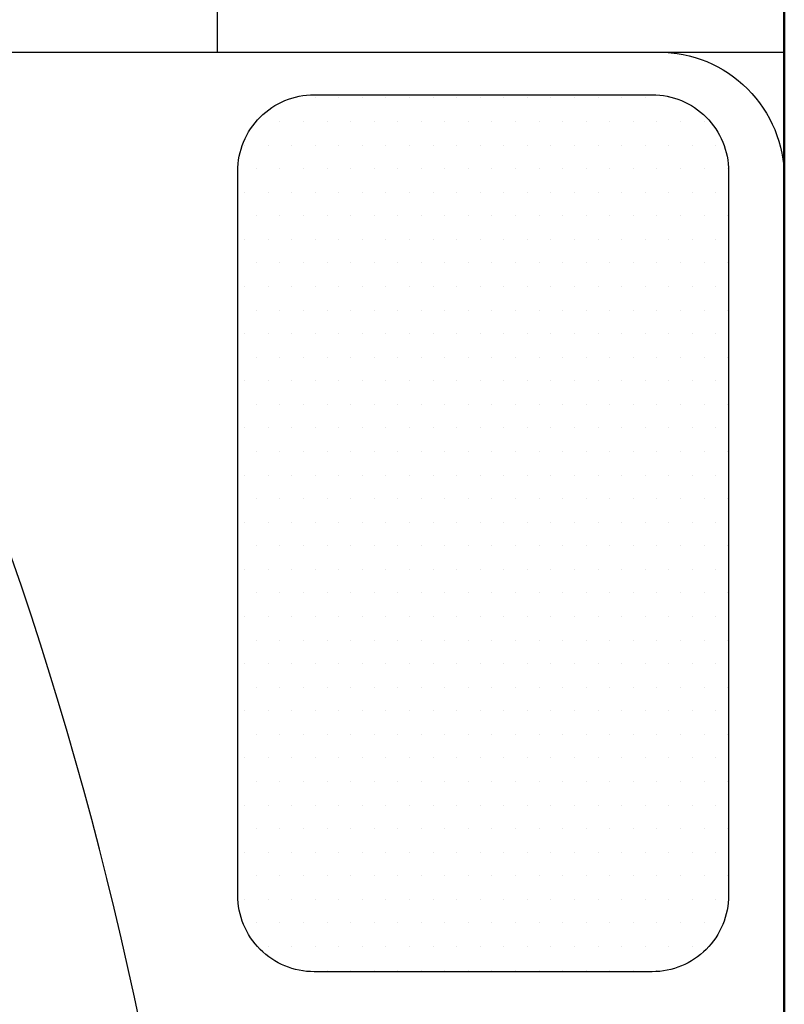
# Model space of a CAD drawing. Units: inches. Extents: x 3064 to 19385, y 846 to 15425.
# Tile 40 of 108: x 5302 to 5326, y 1059 to 1090. Entities that reach past the tile are written whole.
import ezdxf

# ---------------------------------------------------------------- set-up
doc = ezdxf.new("R2010")
doc.units = ezdxf.units.IN
doc.layers.add('A-FLOR-FIXT', color=9, linetype='Continuous', lineweight=18)
doc.layers.add('A-WALL', color=7, linetype='Continuous', lineweight=50)
doc.layers.add('BLOCK', color=6, linetype='Continuous')

# ---------------------------------------------------------------- blocks, each defined once
blk = doc.blocks.new('*X7')
at = {"color": 0}
for p, q in [((266.4375, 457.03125), (266.4375, 457.03125)), ((266.8125, 457.03125), (266.8125, 457.03125)), ((267.1875, 457.03125), (267.1875, 457.03125)), ((267.5625, 457.03125), (267.5625, 457.03125)), ((267.9375, 457.03125), (267.9375, 457.03125)), ((268.3125, 457.03125), (268.3125, 457.03125)), ((268.6875, 457.03125), (268.6875, 457.03125)), ((269.0625, 457.03125), (269.0625, 457.03125)), ((269.4375, 457.03125), (269.4375, 457.03125)), ((269.8125, 457.03125), (269.8125, 457.03125)), ((270.1875, 457.03125), (270.1875, 457.03125)), ((270.5625, 457.03125), (270.5625, 457.03125)), ((270.9375, 457.03125), (270.9375, 457.03125)), ((271.3125, 457.03125), (271.3125, 457.03125)), ((271.6875, 457.03125), (271.6875, 457.03125)), ((272.0625, 457.03125), (272.0625, 457.03125)), ((266.25, 456.9375), (266.25, 456.9375)), ((266.625, 456.9375), (266.625, 456.9375)), ((267, 456.9375), (267, 456.9375)), ((267.375, 456.9375), (267.375, 456.9375)), ((267.75, 456.9375), (267.75, 456.9375)), ((268.125, 456.9375), (268.125, 456.9375)), ((268.5, 456.9375), (268.5, 456.9375)), ((268.875, 456.9375), (268.875, 456.9375)), ((269.25, 456.9375), (269.25, 456.9375)), ((269.625, 456.9375), (269.625, 456.9375)), ((270, 456.9375), (270, 456.9375)), ((270.375, 456.9375), (270.375, 456.9375)), ((270.75, 456.9375), (270.75, 456.9375)), ((271.125, 456.9375), (271.125, 456.9375)), ((271.5, 456.9375), (271.5, 456.9375)), ((271.875, 456.9375), (271.875, 456.9375)), ((272.25, 456.9375), (272.25, 456.9375)), ((266.0625, 456.84375), (266.0625, 456.84375)), ((266.4375, 456.84375), (266.4375, 456.84375)), ((266.8125, 456.84375), (266.8125, 456.84375)), ((267.1875, 456.84375), (267.1875, 456.84375)), ((267.5625, 456.84375), (267.5625, 456.84375)), ((267.9375, 456.84375), (267.9375, 456.84375)), ((268.3125, 456.84375), (268.3125, 456.84375)), ((268.6875, 456.84375), (268.6875, 456.84375)), ((269.0625, 456.84375), (269.0625, 456.84375)), ((269.4375, 456.84375), (269.4375, 456.84375)), ((269.8125, 456.84375), (269.8125, 456.84375)), ((270.1875, 456.84375), (270.1875, 456.84375)), ((270.5625, 456.84375), (270.5625, 456.84375)), ((270.9375, 456.84375), (270.9375, 456.84375)), ((271.3125, 456.84375), (271.3125, 456.84375)), ((271.6875, 456.84375), (271.6875, 456.84375)), ((272.0625, 456.84375), (272.0625, 456.84375)), ((272.4375, 456.84375), (272.4375, 456.84375)), ((266.25, 456.75), (266.25, 456.75)), ((266.625, 456.75), (266.625, 456.75)), ((267, 456.75), (267, 456.75)), ((267.375, 456.75), (267.375, 456.75)), ((267.75, 456.75), (267.75, 456.75)), ((268.125, 456.75), (268.125, 456.75)), ((268.5, 456.75), (268.5, 456.75)), ((268.875, 456.75), (268.875, 456.75)), ((269.25, 456.75), (269.25, 456.75)), ((269.625, 456.75), (269.625, 456.75)), ((270, 456.75), (270, 456.75)), ((270.375, 456.75), (270.375, 456.75)), ((270.75, 456.75), (270.75, 456.75)), ((271.125, 456.75), (271.125, 456.75)), ((271.5, 456.75), (271.5, 456.75)), ((271.875, 456.75), (271.875, 456.75)), ((272.25, 456.75), (272.25, 456.75)), ((272.625, 456.75), (272.625, 456.75)), ((266.0625, 456.65625), (266.0625, 456.65625)), ((266.4375, 456.65625), (266.4375, 456.65625)), ((266.8125, 456.65625), (266.8125, 456.65625)), ((267.1875, 456.65625), (267.1875, 456.65625)), ((267.5625, 456.65625), (267.5625, 456.65625)), ((267.9375, 456.65625), (267.9375, 456.65625)), ((268.3125, 456.65625), (268.3125, 456.65625)), ((268.6875, 456.65625), (268.6875, 456.65625)), ((269.0625, 456.65625), (269.0625, 456.65625)), ((269.4375, 456.65625), (269.4375, 456.65625)), ((269.8125, 456.65625), (269.8125, 456.65625)), ((270.1875, 456.65625), (270.1875, 456.65625)), ((270.5625, 456.65625), (270.5625, 456.65625)), ((270.9375, 456.65625), (270.9375, 456.65625)), ((271.3125, 456.65625), (271.3125, 456.65625)), ((271.6875, 456.65625), (271.6875, 456.65625)), ((272.0625, 456.65625), (272.0625, 456.65625)), ((272.4375, 456.65625), (272.4375, 456.65625)), ((265.875, 456.5625), (265.875, 456.5625)), ((266.25, 456.5625), (266.25, 456.5625)), ((266.625, 456.5625), (266.625, 456.5625)), ((267, 456.5625), (267, 456.5625)), ((267.375, 456.5625), (267.375, 456.5625)), ((267.75, 456.5625), (267.75, 456.5625)), ((268.125, 456.5625), (268.125, 456.5625)), ((268.5, 456.5625), (268.5, 456.5625)), ((268.875, 456.5625), (268.875, 456.5625)), ((269.25, 456.5625), (269.25, 456.5625)), ((269.625, 456.5625), (269.625, 456.5625)), ((270, 456.5625), (270, 456.5625)), ((270.375, 456.5625), (270.375, 456.5625)), ((270.75, 456.5625), (270.75, 456.5625)), ((271.125, 456.5625), (271.125, 456.5625)), ((271.5, 456.5625), (271.5, 456.5625)), ((271.875, 456.5625), (271.875, 456.5625)), ((272.25, 456.5625), (272.25, 456.5625)), ((272.625, 456.5625), (272.625, 456.5625)), ((266.0625, 456.46875), (266.0625, 456.46875)), ((266.4375, 456.46875), (266.4375, 456.46875)), ((266.8125, 456.46875), (266.8125, 456.46875)), ((267.1875, 456.46875), (267.1875, 456.46875)), ((267.5625, 456.46875), (267.5625, 456.46875)), ((267.9375, 456.46875), (267.9375, 456.46875)), ((268.3125, 456.46875), (268.3125, 456.46875)), ((268.6875, 456.46875), (268.6875, 456.46875)), ((269.0625, 456.46875), (269.0625, 456.46875)), ((269.4375, 456.46875), (269.4375, 456.46875)), ((269.8125, 456.46875), (269.8125, 456.46875)), ((270.1875, 456.46875), (270.1875, 456.46875)), ((270.5625, 456.46875), (270.5625, 456.46875)), ((270.9375, 456.46875), (270.9375, 456.46875)), ((271.3125, 456.46875), (271.3125, 456.46875)), ((271.6875, 456.46875), (271.6875, 456.46875)), ((272.0625, 456.46875), (272.0625, 456.46875)), ((272.4375, 456.46875), (272.4375, 456.46875)), ((272.8125, 456.46875), (272.8125, 456.46875)), ((265.875, 456.375), (265.875, 456.375)), ((266.25, 456.375), (266.25, 456.375)), ((266.625, 456.375), (266.625, 456.375)), ((267, 456.375), (267, 456.375)), ((267.375, 456.375), (267.375, 456.375)), ((267.75, 456.375), (267.75, 456.375)), ((268.125, 456.375), (268.125, 456.375)), ((268.5, 456.375), (268.5, 456.375)), ((268.875, 456.375), (268.875, 456.375)), ((269.25, 456.375), (269.25, 456.375)), ((269.625, 456.375), (269.625, 456.375)), ((270, 456.375), (270, 456.375)), ((270.375, 456.375), (270.375, 456.375)), ((270.75, 456.375), (270.75, 456.375)), ((271.125, 456.375), (271.125, 456.375)), ((271.5, 456.375), (271.5, 456.375)), ((271.875, 456.375), (271.875, 456.375)), ((272.25, 456.375), (272.25, 456.375)), ((272.625, 456.375), (272.625, 456.375)), ((266.0625, 456.28125), (266.0625, 456.28125)), ((266.4375, 456.28125), (266.4375, 456.28125)), ((266.8125, 456.28125), (266.8125, 456.28125)), ((267.1875, 456.28125), (267.1875, 456.28125)), ((267.5625, 456.28125), (267.5625, 456.28125)), ((267.9375, 456.28125), (267.9375, 456.28125)), ((268.3125, 456.28125), (268.3125, 456.28125)), ((268.6875, 456.28125), (268.6875, 456.28125)), ((269.0625, 456.28125), (269.0625, 456.28125)), ((269.4375, 456.28125), (269.4375, 456.28125)), ((269.8125, 456.28125), (269.8125, 456.28125)), ((270.1875, 456.28125), (270.1875, 456.28125)), ((270.5625, 456.28125), (270.5625, 456.28125)), ((270.9375, 456.28125), (270.9375, 456.28125)), ((271.3125, 456.28125), (271.3125, 456.28125)), ((271.6875, 456.28125), (271.6875, 456.28125)), ((272.0625, 456.28125), (272.0625, 456.28125)), ((272.4375, 456.28125), (272.4375, 456.28125)), ((272.8125, 456.28125), (272.8125, 456.28125)), ((265.875, 456.1875), (265.875, 456.1875)), ((266.25, 456.1875), (266.25, 456.1875)), ((266.625, 456.1875), (266.625, 456.1875)), ((267, 456.1875), (267, 456.1875)), ((267.375, 456.1875), (267.375, 456.1875)), ((267.75, 456.1875), (267.75, 456.1875)), ((268.125, 456.1875), (268.125, 456.1875)), ((268.5, 456.1875), (268.5, 456.1875)), ((268.875, 456.1875), (268.875, 456.1875)), ((269.25, 456.1875), (269.25, 456.1875)), ((269.625, 456.1875), (269.625, 456.1875)), ((270, 456.1875), (270, 456.1875)), ((270.375, 456.1875), (270.375, 456.1875)), ((270.75, 456.1875), (270.75, 456.1875)), ((271.125, 456.1875), (271.125, 456.1875)), ((271.5, 456.1875), (271.5, 456.1875)), ((271.875, 456.1875), (271.875, 456.1875)), ((272.25, 456.1875), (272.25, 456.1875)), ((272.625, 456.1875), (272.625, 456.1875)), ((266.0625, 456.09375), (266.0625, 456.09375)), ((266.4375, 456.09375), (266.4375, 456.09375)), ((266.8125, 456.09375), (266.8125, 456.09375)), ((267.1875, 456.09375), (267.1875, 456.09375)), ((267.5625, 456.09375), (267.5625, 456.09375)), ((267.9375, 456.09375), (267.9375, 456.09375)), ((268.3125, 456.09375), (268.3125, 456.09375)), ((268.6875, 456.09375), (268.6875, 456.09375)), ((269.0625, 456.09375), (269.0625, 456.09375)), ((269.4375, 456.09375), (269.4375, 456.09375)), ((269.8125, 456.09375), (269.8125, 456.09375)), ((270.1875, 456.09375), (270.1875, 456.09375)), ((270.5625, 456.09375), (270.5625, 456.09375)), ((270.9375, 456.09375), (270.9375, 456.09375)), ((271.3125, 456.09375), (271.3125, 456.09375)), ((271.6875, 456.09375), (271.6875, 456.09375)), ((272.0625, 456.09375), (272.0625, 456.09375)), ((272.4375, 456.09375), (272.4375, 456.09375)), ((272.8125, 456.09375), (272.8125, 456.09375)), ((265.875, 456), (265.875, 456)), ((266.25, 456), (266.25, 456)), ((266.625, 456), (266.625, 456)), ((267, 456), (267, 456)), ((267.375, 456), (267.375, 456)), ((267.75, 456), (267.75, 456)), ((268.125, 456), (268.125, 456)), ((268.5, 456), (268.5, 456)), ((268.875, 456), (268.875, 456)), ((269.25, 456), (269.25, 456)), ((269.625, 456), (269.625, 456)), ((270, 456), (270, 456)), ((270.375, 456), (270.375, 456)), ((270.75, 456), (270.75, 456)), ((271.125, 456), (271.125, 456)), ((271.5, 456), (271.5, 456)), ((271.875, 456), (271.875, 456)), ((272.25, 456), (272.25, 456)), ((272.625, 456), (272.625, 456)), ((266.0625, 455.90625), (266.0625, 455.90625)), ((266.4375, 455.90625), (266.4375, 455.90625)), ((266.8125, 455.90625), (266.8125, 455.90625)), ((267.1875, 455.90625), (267.1875, 455.90625)), ((267.5625, 455.90625), (267.5625, 455.90625)), ((267.9375, 455.90625), (267.9375, 455.90625)), ((268.3125, 455.90625), (268.3125, 455.90625)), ((268.6875, 455.90625), (268.6875, 455.90625)), ((269.0625, 455.90625), (269.0625, 455.90625)), ((269.4375, 455.90625), (269.4375, 455.90625)), ((269.8125, 455.90625), (269.8125, 455.90625)), ((270.1875, 455.90625), (270.1875, 455.90625)), ((270.5625, 455.90625), (270.5625, 455.90625)), ((270.9375, 455.90625), (270.9375, 455.90625)), ((271.3125, 455.90625), (271.3125, 455.90625)), ((271.6875, 455.90625), (271.6875, 455.90625)), ((272.0625, 455.90625), (272.0625, 455.90625)), ((272.4375, 455.90625), (272.4375, 455.90625)), ((272.8125, 455.90625), (272.8125, 455.90625)), ((265.875, 455.8125), (265.875, 455.8125)), ((266.25, 455.8125), (266.25, 455.8125)), ((266.625, 455.8125), (266.625, 455.8125)), ((267, 455.8125), (267, 455.8125)), ((267.375, 455.8125), (267.375, 455.8125)), ((267.75, 455.8125), (267.75, 455.8125)), ((268.125, 455.8125), (268.125, 455.8125)), ((268.5, 455.8125), (268.5, 455.8125)), ((268.875, 455.8125), (268.875, 455.8125)), ((269.25, 455.8125), (269.25, 455.8125)), ((269.625, 455.8125), (269.625, 455.8125)), ((270, 455.8125), (270, 455.8125)), ((270.375, 455.8125), (270.375, 455.8125)), ((270.75, 455.8125), (270.75, 455.8125)), ((271.125, 455.8125), (271.125, 455.8125)), ((271.5, 455.8125), (271.5, 455.8125)), ((271.875, 455.8125), (271.875, 455.8125)), ((272.25, 455.8125), (272.25, 455.8125)), ((272.625, 455.8125), (272.625, 455.8125)), ((266.0625, 455.71875), (266.0625, 455.71875)), ((266.4375, 455.71875), (266.4375, 455.71875)), ((266.8125, 455.71875), (266.8125, 455.71875)), ((267.1875, 455.71875), (267.1875, 455.71875)), ((267.5625, 455.71875), (267.5625, 455.71875)), ((267.9375, 455.71875), (267.9375, 455.71875)), ((268.3125, 455.71875), (268.3125, 455.71875)), ((268.6875, 455.71875), (268.6875, 455.71875)), ((269.0625, 455.71875), (269.0625, 455.71875)), ((269.4375, 455.71875), (269.4375, 455.71875)), ((269.8125, 455.71875), (269.8125, 455.71875)), ((270.1875, 455.71875), (270.1875, 455.71875)), ((270.5625, 455.71875), (270.5625, 455.71875)), ((270.9375, 455.71875), (270.9375, 455.71875)), ((271.3125, 455.71875), (271.3125, 455.71875)), ((271.6875, 455.71875), (271.6875, 455.71875)), ((272.0625, 455.71875), (272.0625, 455.71875)), ((272.4375, 455.71875), (272.4375, 455.71875)), ((272.8125, 455.71875), (272.8125, 455.71875)), ((265.875, 455.625), (265.875, 455.625)), ((266.25, 455.625), (266.25, 455.625)), ((266.625, 455.625), (266.625, 455.625)), ((267, 455.625), (267, 455.625)), ((267.375, 455.625), (267.375, 455.625)), ((267.75, 455.625), (267.75, 455.625)), ((268.125, 455.625), (268.125, 455.625)), ((268.5, 455.625), (268.5, 455.625)), ((268.875, 455.625), (268.875, 455.625)), ((269.25, 455.625), (269.25, 455.625)), ((269.625, 455.625), (269.625, 455.625)), ((270, 455.625), (270, 455.625)), ((270.375, 455.625), (270.375, 455.625)), ((270.75, 455.625), (270.75, 455.625)), ((271.125, 455.625), (271.125, 455.625)), ((271.5, 455.625), (271.5, 455.625)), ((271.875, 455.625), (271.875, 455.625)), ((272.25, 455.625), (272.25, 455.625)), ((272.625, 455.625), (272.625, 455.625)), ((266.0625, 455.53125), (266.0625, 455.53125)), ((266.4375, 455.53125), (266.4375, 455.53125)), ((266.8125, 455.53125), (266.8125, 455.53125)), ((267.1875, 455.53125), (267.1875, 455.53125)), ((267.5625, 455.53125), (267.5625, 455.53125)), ((267.9375, 455.53125), (267.9375, 455.53125)), ((268.3125, 455.53125), (268.3125, 455.53125)), ((268.6875, 455.53125), (268.6875, 455.53125)), ((269.0625, 455.53125), (269.0625, 455.53125)), ((269.4375, 455.53125), (269.4375, 455.53125)), ((269.8125, 455.53125), (269.8125, 455.53125)), ((270.1875, 455.53125), (270.1875, 455.53125)), ((270.5625, 455.53125), (270.5625, 455.53125)), ((270.9375, 455.53125), (270.9375, 455.53125)), ((271.3125, 455.53125), (271.3125, 455.53125)), ((271.6875, 455.53125), (271.6875, 455.53125)), ((272.0625, 455.53125), (272.0625, 455.53125)), ((272.4375, 455.53125), (272.4375, 455.53125)), ((272.8125, 455.53125), (272.8125, 455.53125)), ((265.875, 455.4375), (265.875, 455.4375)), ((266.25, 455.4375), (266.25, 455.4375)), ((266.625, 455.4375), (266.625, 455.4375)), ((267, 455.4375), (267, 455.4375)), ((267.375, 455.4375), (267.375, 455.4375)), ((267.75, 455.4375), (267.75, 455.4375)), ((268.125, 455.4375), (268.125, 455.4375)), ((268.5, 455.4375), (268.5, 455.4375)), ((268.875, 455.4375), (268.875, 455.4375)), ((269.25, 455.4375), (269.25, 455.4375)), ((269.625, 455.4375), (269.625, 455.4375)), ((270, 455.4375), (270, 455.4375)), ((270.375, 455.4375), (270.375, 455.4375)), ((270.75, 455.4375), (270.75, 455.4375)), ((271.125, 455.4375), (271.125, 455.4375)), ((271.5, 455.4375), (271.5, 455.4375)), ((271.875, 455.4375), (271.875, 455.4375)), ((272.25, 455.4375), (272.25, 455.4375)), ((272.625, 455.4375), (272.625, 455.4375)), ((266.0625, 455.34375), (266.0625, 455.34375)), ((266.4375, 455.34375), (266.4375, 455.34375)), ((266.8125, 455.34375), (266.8125, 455.34375)), ((267.1875, 455.34375), (267.1875, 455.34375)), ((267.5625, 455.34375), (267.5625, 455.34375)), ((267.9375, 455.34375), (267.9375, 455.34375)), ((268.3125, 455.34375), (268.3125, 455.34375)), ((268.6875, 455.34375), (268.6875, 455.34375)), ((269.0625, 455.34375), (269.0625, 455.34375)), ((269.4375, 455.34375), (269.4375, 455.34375)), ((269.8125, 455.34375), (269.8125, 455.34375)), ((270.1875, 455.34375), (270.1875, 455.34375)), ((270.5625, 455.34375), (270.5625, 455.34375)), ((270.9375, 455.34375), (270.9375, 455.34375)), ((271.3125, 455.34375), (271.3125, 455.34375)), ((271.6875, 455.34375), (271.6875, 455.34375)), ((272.0625, 455.34375), (272.0625, 455.34375)), ((272.4375, 455.34375), (272.4375, 455.34375)), ((272.8125, 455.34375), (272.8125, 455.34375)), ((265.875, 455.25), (265.875, 455.25)), ((266.25, 455.25), (266.25, 455.25)), ((266.625, 455.25), (266.625, 455.25)), ((267, 455.25), (267, 455.25)), ((267.375, 455.25), (267.375, 455.25)), ((267.75, 455.25), (267.75, 455.25)), ((268.125, 455.25), (268.125, 455.25)), ((268.5, 455.25), (268.5, 455.25)), ((268.875, 455.25), (268.875, 455.25)), ((269.25, 455.25), (269.25, 455.25)), ((269.625, 455.25), (269.625, 455.25)), ((270, 455.25), (270, 455.25)), ((270.375, 455.25), (270.375, 455.25)), ((270.75, 455.25), (270.75, 455.25)), ((271.125, 455.25), (271.125, 455.25)), ((271.5, 455.25), (271.5, 455.25)), ((271.875, 455.25), (271.875, 455.25)), ((272.25, 455.25), (272.25, 455.25)), ((272.625, 455.25), (272.625, 455.25)), ((266.0625, 455.15625), (266.0625, 455.15625)), ((266.4375, 455.15625), (266.4375, 455.15625)), ((266.8125, 455.15625), (266.8125, 455.15625)), ((267.1875, 455.15625), (267.1875, 455.15625)), ((267.5625, 455.15625), (267.5625, 455.15625)), ((267.9375, 455.15625), (267.9375, 455.15625)), ((268.3125, 455.15625), (268.3125, 455.15625)), ((268.6875, 455.15625), (268.6875, 455.15625)), ((269.0625, 455.15625), (269.0625, 455.15625)), ((269.4375, 455.15625), (269.4375, 455.15625)), ((269.8125, 455.15625), (269.8125, 455.15625)), ((270.1875, 455.15625), (270.1875, 455.15625)), ((270.5625, 455.15625), (270.5625, 455.15625)), ((270.9375, 455.15625), (270.9375, 455.15625)), ((271.3125, 455.15625), (271.3125, 455.15625)), ((271.6875, 455.15625), (271.6875, 455.15625)), ((272.0625, 455.15625), (272.0625, 455.15625)), ((272.4375, 455.15625), (272.4375, 455.15625)), ((272.8125, 455.15625), (272.8125, 455.15625)), ((265.875, 455.0625), (265.875, 455.0625)), ((266.25, 455.0625), (266.25, 455.0625)), ((266.625, 455.0625), (266.625, 455.0625)), ((267, 455.0625), (267, 455.0625)), ((267.375, 455.0625), (267.375, 455.0625)), ((267.75, 455.0625), (267.75, 455.0625)), ((268.125, 455.0625), (268.125, 455.0625)), ((268.5, 455.0625), (268.5, 455.0625)), ((268.875, 455.0625), (268.875, 455.0625)), ((269.25, 455.0625), (269.25, 455.0625)), ((269.625, 455.0625), (269.625, 455.0625)), ((270, 455.0625), (270, 455.0625)), ((270.375, 455.0625), (270.375, 455.0625)), ((270.75, 455.0625), (270.75, 455.0625)), ((271.125, 455.0625), (271.125, 455.0625)), ((271.5, 455.0625), (271.5, 455.0625)), ((271.875, 455.0625), (271.875, 455.0625)), ((272.25, 455.0625), (272.25, 455.0625)), ((272.625, 455.0625), (272.625, 455.0625)), ((266.0625, 454.96875), (266.0625, 454.96875)), ((266.4375, 454.96875), (266.4375, 454.96875)), ((266.8125, 454.96875), (266.8125, 454.96875)), ((267.1875, 454.96875), (267.1875, 454.96875)), ((267.5625, 454.96875), (267.5625, 454.96875)), ((267.9375, 454.96875), (267.9375, 454.96875)), ((268.3125, 454.96875), (268.3125, 454.96875)), ((268.6875, 454.96875), (268.6875, 454.96875)), ((269.0625, 454.96875), (269.0625, 454.96875)), ((269.4375, 454.96875), (269.4375, 454.96875)), ((269.8125, 454.96875), (269.8125, 454.96875)), ((270.1875, 454.96875), (270.1875, 454.96875)), ((270.5625, 454.96875), (270.5625, 454.96875)), ((270.9375, 454.96875), (270.9375, 454.96875)), ((271.3125, 454.96875), (271.3125, 454.96875)), ((271.6875, 454.96875), (271.6875, 454.96875)), ((272.0625, 454.96875), (272.0625, 454.96875)), ((272.4375, 454.96875), (272.4375, 454.96875)), ((272.8125, 454.96875), (272.8125, 454.96875)), ((265.875, 454.875), (265.875, 454.875)), ((266.25, 454.875), (266.25, 454.875)), ((266.625, 454.875), (266.625, 454.875)), ((267, 454.875), (267, 454.875)), ((267.375, 454.875), (267.375, 454.875)), ((267.75, 454.875), (267.75, 454.875)), ((268.125, 454.875), (268.125, 454.875)), ((268.5, 454.875), (268.5, 454.875)), ((268.875, 454.875), (268.875, 454.875)), ((269.25, 454.875), (269.25, 454.875)), ((269.625, 454.875), (269.625, 454.875)), ((270, 454.875), (270, 454.875)), ((270.375, 454.875), (270.375, 454.875)), ((270.75, 454.875), (270.75, 454.875)), ((271.125, 454.875), (271.125, 454.875)), ((271.5, 454.875), (271.5, 454.875)), ((271.875, 454.875), (271.875, 454.875)), ((272.25, 454.875), (272.25, 454.875)), ((272.625, 454.875), (272.625, 454.875)), ((266.0625, 454.78125), (266.0625, 454.78125)), ((266.4375, 454.78125), (266.4375, 454.78125)), ((266.8125, 454.78125), (266.8125, 454.78125)), ((267.1875, 454.78125), (267.1875, 454.78125)), ((267.5625, 454.78125), (267.5625, 454.78125)), ((267.9375, 454.78125), (267.9375, 454.78125)), ((268.3125, 454.78125), (268.3125, 454.78125)), ((268.6875, 454.78125), (268.6875, 454.78125)), ((269.0625, 454.78125), (269.0625, 454.78125)), ((269.4375, 454.78125), (269.4375, 454.78125)), ((269.8125, 454.78125), (269.8125, 454.78125)), ((270.1875, 454.78125), (270.1875, 454.78125)), ((270.5625, 454.78125), (270.5625, 454.78125)), ((270.9375, 454.78125), (270.9375, 454.78125)), ((271.3125, 454.78125), (271.3125, 454.78125)), ((271.6875, 454.78125), (271.6875, 454.78125)), ((272.0625, 454.78125), (272.0625, 454.78125)), ((272.4375, 454.78125), (272.4375, 454.78125)), ((272.8125, 454.78125), (272.8125, 454.78125)), ((265.875, 454.6875), (265.875, 454.6875)), ((266.25, 454.6875), (266.25, 454.6875)), ((266.625, 454.6875), (266.625, 454.6875)), ((267, 454.6875), (267, 454.6875)), ((267.375, 454.6875), (267.375, 454.6875)), ((267.75, 454.6875), (267.75, 454.6875)), ((268.125, 454.6875), (268.125, 454.6875)), ((268.5, 454.6875), (268.5, 454.6875)), ((268.875, 454.6875), (268.875, 454.6875)), ((269.25, 454.6875), (269.25, 454.6875)), ((269.625, 454.6875), (269.625, 454.6875)), ((270, 454.6875), (270, 454.6875)), ((270.375, 454.6875), (270.375, 454.6875)), ((270.75, 454.6875), (270.75, 454.6875)), ((271.125, 454.6875), (271.125, 454.6875)), ((271.5, 454.6875), (271.5, 454.6875)), ((271.875, 454.6875), (271.875, 454.6875)), ((272.25, 454.6875), (272.25, 454.6875)), ((272.625, 454.6875), (272.625, 454.6875)), ((266.0625, 454.59375), (266.0625, 454.59375)), ((266.4375, 454.59375), (266.4375, 454.59375)), ((266.8125, 454.59375), (266.8125, 454.59375)), ((267.1875, 454.59375), (267.1875, 454.59375)), ((267.5625, 454.59375), (267.5625, 454.59375)), ((267.9375, 454.59375), (267.9375, 454.59375)), ((268.3125, 454.59375), (268.3125, 454.59375)), ((268.6875, 454.59375), (268.6875, 454.59375)), ((269.0625, 454.59375), (269.0625, 454.59375)), ((269.4375, 454.59375), (269.4375, 454.59375)), ((269.8125, 454.59375), (269.8125, 454.59375)), ((270.1875, 454.59375), (270.1875, 454.59375)), ((270.5625, 454.59375), (270.5625, 454.59375)), ((270.9375, 454.59375), (270.9375, 454.59375)), ((271.3125, 454.59375), (271.3125, 454.59375)), ((271.6875, 454.59375), (271.6875, 454.59375)), ((272.0625, 454.59375), (272.0625, 454.59375)), ((272.4375, 454.59375), (272.4375, 454.59375)), ((272.8125, 454.59375), (272.8125, 454.59375)), ((265.875, 454.5), (265.875, 454.5)), ((266.25, 454.5), (266.25, 454.5)), ((266.625, 454.5), (266.625, 454.5)), ((267, 454.5), (267, 454.5)), ((267.375, 454.5), (267.375, 454.5)), ((267.75, 454.5), (267.75, 454.5)), ((268.125, 454.5), (268.125, 454.5)), ((268.5, 454.5), (268.5, 454.5)), ((268.875, 454.5), (268.875, 454.5)), ((269.25, 454.5), (269.25, 454.5)), ((269.625, 454.5), (269.625, 454.5)), ((270, 454.5), (270, 454.5)), ((270.375, 454.5), (270.375, 454.5)), ((270.75, 454.5), (270.75, 454.5)), ((271.125, 454.5), (271.125, 454.5)), ((271.5, 454.5), (271.5, 454.5)), ((271.875, 454.5), (271.875, 454.5)), ((272.25, 454.5), (272.25, 454.5)), ((272.625, 454.5), (272.625, 454.5)), ((266.0625, 454.40625), (266.0625, 454.40625)), ((266.4375, 454.40625), (266.4375, 454.40625)), ((266.8125, 454.40625), (266.8125, 454.40625)), ((267.1875, 454.40625), (267.1875, 454.40625)), ((267.5625, 454.40625), (267.5625, 454.40625)), ((267.9375, 454.40625), (267.9375, 454.40625)), ((268.3125, 454.40625), (268.3125, 454.40625)), ((268.6875, 454.40625), (268.6875, 454.40625)), ((269.0625, 454.40625), (269.0625, 454.40625)), ((269.4375, 454.40625), (269.4375, 454.40625)), ((269.8125, 454.40625), (269.8125, 454.40625)), ((270.1875, 454.40625), (270.1875, 454.40625)), ((270.5625, 454.40625), (270.5625, 454.40625)), ((270.9375, 454.40625), (270.9375, 454.40625)), ((271.3125, 454.40625), (271.3125, 454.40625)), ((271.6875, 454.40625), (271.6875, 454.40625)), ((272.0625, 454.40625), (272.0625, 454.40625)), ((272.4375, 454.40625), (272.4375, 454.40625)), ((272.8125, 454.40625), (272.8125, 454.40625)), ((265.875, 454.3125), (265.875, 454.3125)), ((266.25, 454.3125), (266.25, 454.3125)), ((266.625, 454.3125), (266.625, 454.3125)), ((267, 454.3125), (267, 454.3125)), ((267.375, 454.3125), (267.375, 454.3125)), ((267.75, 454.3125), (267.75, 454.3125)), ((268.125, 454.3125), (268.125, 454.3125)), ((268.5, 454.3125), (268.5, 454.3125)), ((268.875, 454.3125), (268.875, 454.3125)), ((269.25, 454.3125), (269.25, 454.3125)), ((269.625, 454.3125), (269.625, 454.3125)), ((270, 454.3125), (270, 454.3125)), ((270.375, 454.3125), (270.375, 454.3125)), ((270.75, 454.3125), (270.75, 454.3125)), ((271.125, 454.3125), (271.125, 454.3125)), ((271.5, 454.3125), (271.5, 454.3125)), ((271.875, 454.3125), (271.875, 454.3125)), ((272.25, 454.3125), (272.25, 454.3125)), ((272.625, 454.3125), (272.625, 454.3125)), ((266.0625, 454.21875), (266.0625, 454.21875)), ((266.4375, 454.21875), (266.4375, 454.21875)), ((266.8125, 454.21875), (266.8125, 454.21875)), ((267.1875, 454.21875), (267.1875, 454.21875)), ((267.5625, 454.21875), (267.5625, 454.21875)), ((267.9375, 454.21875), (267.9375, 454.21875)), ((268.3125, 454.21875), (268.3125, 454.21875)), ((268.6875, 454.21875), (268.6875, 454.21875)), ((269.0625, 454.21875), (269.0625, 454.21875)), ((269.4375, 454.21875), (269.4375, 454.21875)), ((269.8125, 454.21875), (269.8125, 454.21875)), ((270.1875, 454.21875), (270.1875, 454.21875)), ((270.5625, 454.21875), (270.5625, 454.21875)), ((270.9375, 454.21875), (270.9375, 454.21875)), ((271.3125, 454.21875), (271.3125, 454.21875)), ((271.6875, 454.21875), (271.6875, 454.21875)), ((272.0625, 454.21875), (272.0625, 454.21875)), ((272.4375, 454.21875), (272.4375, 454.21875)), ((272.8125, 454.21875), (272.8125, 454.21875)), ((265.875, 454.125), (265.875, 454.125)), ((266.25, 454.125), (266.25, 454.125)), ((266.625, 454.125), (266.625, 454.125)), ((267, 454.125), (267, 454.125)), ((267.375, 454.125), (267.375, 454.125)), ((267.75, 454.125), (267.75, 454.125)), ((268.125, 454.125), (268.125, 454.125)), ((268.5, 454.125), (268.5, 454.125)), ((268.875, 454.125), (268.875, 454.125)), ((269.25, 454.125), (269.25, 454.125)), ((269.625, 454.125), (269.625, 454.125)), ((270, 454.125), (270, 454.125)), ((270.375, 454.125), (270.375, 454.125)), ((270.75, 454.125), (270.75, 454.125)), ((271.125, 454.125), (271.125, 454.125)), ((271.5, 454.125), (271.5, 454.125)), ((271.875, 454.125), (271.875, 454.125)), ((272.25, 454.125), (272.25, 454.125)), ((272.625, 454.125), (272.625, 454.125)), ((266.0625, 454.03125), (266.0625, 454.03125)), ((266.4375, 454.03125), (266.4375, 454.03125)), ((266.8125, 454.03125), (266.8125, 454.03125)), ((267.1875, 454.03125), (267.1875, 454.03125)), ((267.5625, 454.03125), (267.5625, 454.03125)), ((267.9375, 454.03125), (267.9375, 454.03125)), ((268.3125, 454.03125), (268.3125, 454.03125)), ((268.6875, 454.03125), (268.6875, 454.03125)), ((269.0625, 454.03125), (269.0625, 454.03125)), ((269.4375, 454.03125), (269.4375, 454.03125)), ((269.8125, 454.03125), (269.8125, 454.03125)), ((270.1875, 454.03125), (270.1875, 454.03125)), ((270.5625, 454.03125), (270.5625, 454.03125)), ((270.9375, 454.03125), (270.9375, 454.03125)), ((271.3125, 454.03125), (271.3125, 454.03125)), ((271.6875, 454.03125), (271.6875, 454.03125)), ((272.0625, 454.03125), (272.0625, 454.03125)), ((272.4375, 454.03125), (272.4375, 454.03125)), ((272.8125, 454.03125), (272.8125, 454.03125)), ((265.875, 453.9375), (265.875, 453.9375)), ((266.25, 453.9375), (266.25, 453.9375)), ((266.625, 453.9375), (266.625, 453.9375)), ((267, 453.9375), (267, 453.9375)), ((267.375, 453.9375), (267.375, 453.9375)), ((267.75, 453.9375), (267.75, 453.9375)), ((268.125, 453.9375), (268.125, 453.9375)), ((268.5, 453.9375), (268.5, 453.9375)), ((268.875, 453.9375), (268.875, 453.9375)), ((269.25, 453.9375), (269.25, 453.9375)), ((269.625, 453.9375), (269.625, 453.9375)), ((270, 453.9375), (270, 453.9375)), ((270.375, 453.9375), (270.375, 453.9375)), ((270.75, 453.9375), (270.75, 453.9375)), ((271.125, 453.9375), (271.125, 453.9375)), ((271.5, 453.9375), (271.5, 453.9375)), ((271.875, 453.9375), (271.875, 453.9375)), ((272.25, 453.9375), (272.25, 453.9375)), ((272.625, 453.9375), (272.625, 453.9375)), ((266.0625, 453.84375), (266.0625, 453.84375)), ((266.4375, 453.84375), (266.4375, 453.84375)), ((266.8125, 453.84375), (266.8125, 453.84375)), ((267.1875, 453.84375), (267.1875, 453.84375)), ((267.5625, 453.84375), (267.5625, 453.84375)), ((267.9375, 453.84375), (267.9375, 453.84375)), ((268.3125, 453.84375), (268.3125, 453.84375)), ((268.6875, 453.84375), (268.6875, 453.84375)), ((269.0625, 453.84375), (269.0625, 453.84375)), ((269.4375, 453.84375), (269.4375, 453.84375)), ((269.8125, 453.84375), (269.8125, 453.84375)), ((270.1875, 453.84375), (270.1875, 453.84375)), ((270.5625, 453.84375), (270.5625, 453.84375)), ((270.9375, 453.84375), (270.9375, 453.84375)), ((271.3125, 453.84375), (271.3125, 453.84375)), ((271.6875, 453.84375), (271.6875, 453.84375)), ((272.0625, 453.84375), (272.0625, 453.84375)), ((272.4375, 453.84375), (272.4375, 453.84375)), ((272.8125, 453.84375), (272.8125, 453.84375)), ((265.875, 453.75), (265.875, 453.75)), ((266.25, 453.75), (266.25, 453.75)), ((266.625, 453.75), (266.625, 453.75)), ((267, 453.75), (267, 453.75)), ((267.375, 453.75), (267.375, 453.75)), ((267.75, 453.75), (267.75, 453.75)), ((268.125, 453.75), (268.125, 453.75)), ((268.5, 453.75), (268.5, 453.75)), ((268.875, 453.75), (268.875, 453.75)), ((269.25, 453.75), (269.25, 453.75)), ((269.625, 453.75), (269.625, 453.75)), ((270, 453.75), (270, 453.75)), ((270.375, 453.75), (270.375, 453.75)), ((270.75, 453.75), (270.75, 453.75)), ((271.125, 453.75), (271.125, 453.75)), ((271.5, 453.75), (271.5, 453.75)), ((271.875, 453.75), (271.875, 453.75)), ((272.25, 453.75), (272.25, 453.75)), ((272.625, 453.75), (272.625, 453.75)), ((266.0625, 453.65625), (266.0625, 453.65625)), ((266.4375, 453.65625), (266.4375, 453.65625)), ((266.8125, 453.65625), (266.8125, 453.65625)), ((267.1875, 453.65625), (267.1875, 453.65625)), ((267.5625, 453.65625), (267.5625, 453.65625)), ((267.9375, 453.65625), (267.9375, 453.65625)), ((268.3125, 453.65625), (268.3125, 453.65625)), ((268.6875, 453.65625), (268.6875, 453.65625)), ((269.0625, 453.65625), (269.0625, 453.65625)), ((269.4375, 453.65625), (269.4375, 453.65625)), ((269.8125, 453.65625), (269.8125, 453.65625)), ((270.1875, 453.65625), (270.1875, 453.65625)), ((270.5625, 453.65625), (270.5625, 453.65625)), ((270.9375, 453.65625), (270.9375, 453.65625)), ((271.3125, 453.65625), (271.3125, 453.65625)), ((271.6875, 453.65625), (271.6875, 453.65625)), ((272.0625, 453.65625), (272.0625, 453.65625)), ((272.4375, 453.65625), (272.4375, 453.65625)), ((272.8125, 453.65625), (272.8125, 453.65625)), ((266.25, 453.5625), (266.25, 453.5625)), ((266.625, 453.5625), (266.625, 453.5625)), ((267, 453.5625), (267, 453.5625)), ((267.375, 453.5625), (267.375, 453.5625)), ((267.75, 453.5625), (267.75, 453.5625)), ((268.125, 453.5625), (268.125, 453.5625)), ((268.5, 453.5625), (268.5, 453.5625)), ((268.875, 453.5625), (268.875, 453.5625)), ((269.25, 453.5625), (269.25, 453.5625)), ((269.625, 453.5625), (269.625, 453.5625)), ((270, 453.5625), (270, 453.5625)), ((270.375, 453.5625), (270.375, 453.5625)), ((270.75, 453.5625), (270.75, 453.5625)), ((271.125, 453.5625), (271.125, 453.5625)), ((271.5, 453.5625), (271.5, 453.5625)), ((271.875, 453.5625), (271.875, 453.5625)), ((272.25, 453.5625), (272.25, 453.5625)), ((272.625, 453.5625), (272.625, 453.5625)), ((266.0625, 453.46875), (266.0625, 453.46875)), ((266.4375, 453.46875), (266.4375, 453.46875)), ((266.8125, 453.46875), (266.8125, 453.46875)), ((267.1875, 453.46875), (267.1875, 453.46875)), ((267.5625, 453.46875), (267.5625, 453.46875)), ((267.9375, 453.46875), (267.9375, 453.46875)), ((268.3125, 453.46875), (268.3125, 453.46875)), ((268.6875, 453.46875), (268.6875, 453.46875)), ((269.0625, 453.46875), (269.0625, 453.46875)), ((269.4375, 453.46875), (269.4375, 453.46875)), ((269.8125, 453.46875), (269.8125, 453.46875)), ((270.1875, 453.46875), (270.1875, 453.46875)), ((270.5625, 453.46875), (270.5625, 453.46875)), ((270.9375, 453.46875), (270.9375, 453.46875)), ((271.3125, 453.46875), (271.3125, 453.46875)), ((271.6875, 453.46875), (271.6875, 453.46875)), ((272.0625, 453.46875), (272.0625, 453.46875)), ((272.4375, 453.46875), (272.4375, 453.46875)), ((266.25, 453.375), (266.25, 453.375)), ((266.625, 453.375), (266.625, 453.375)), ((267, 453.375), (267, 453.375)), ((267.375, 453.375), (267.375, 453.375)), ((267.75, 453.375), (267.75, 453.375)), ((268.125, 453.375), (268.125, 453.375)), ((268.5, 453.375), (268.5, 453.375)), ((268.875, 453.375), (268.875, 453.375)), ((269.25, 453.375), (269.25, 453.375)), ((269.625, 453.375), (269.625, 453.375)), ((270, 453.375), (270, 453.375)), ((270.375, 453.375), (270.375, 453.375)), ((270.75, 453.375), (270.75, 453.375)), ((271.125, 453.375), (271.125, 453.375)), ((271.5, 453.375), (271.5, 453.375)), ((271.875, 453.375), (271.875, 453.375)), ((272.25, 453.375), (272.25, 453.375)), ((272.625, 453.375), (272.625, 453.375)), ((266.0625, 453.28125), (266.0625, 453.28125)), ((266.4375, 453.28125), (266.4375, 453.28125)), ((266.8125, 453.28125), (266.8125, 453.28125)), ((267.1875, 453.28125), (267.1875, 453.28125)), ((267.5625, 453.28125), (267.5625, 453.28125)), ((267.9375, 453.28125), (267.9375, 453.28125)), ((268.3125, 453.28125), (268.3125, 453.28125)), ((268.6875, 453.28125), (268.6875, 453.28125)), ((269.0625, 453.28125), (269.0625, 453.28125)), ((269.4375, 453.28125), (269.4375, 453.28125)), ((269.8125, 453.28125), (269.8125, 453.28125)), ((270.1875, 453.28125), (270.1875, 453.28125)), ((270.5625, 453.28125), (270.5625, 453.28125)), ((270.9375, 453.28125), (270.9375, 453.28125)), ((271.3125, 453.28125), (271.3125, 453.28125)), ((271.6875, 453.28125), (271.6875, 453.28125)), ((272.0625, 453.28125), (272.0625, 453.28125)), ((272.4375, 453.28125), (272.4375, 453.28125)), ((266.25, 453.1875), (266.25, 453.1875)), ((266.625, 453.1875), (266.625, 453.1875)), ((267, 453.1875), (267, 453.1875)), ((267.375, 453.1875), (267.375, 453.1875)), ((267.75, 453.1875), (267.75, 453.1875)), ((268.125, 453.1875), (268.125, 453.1875)), ((268.5, 453.1875), (268.5, 453.1875)), ((268.875, 453.1875), (268.875, 453.1875)), ((269.25, 453.1875), (269.25, 453.1875)), ((269.625, 453.1875), (269.625, 453.1875)), ((270, 453.1875), (270, 453.1875)), ((270.375, 453.1875), (270.375, 453.1875)), ((270.75, 453.1875), (270.75, 453.1875)), ((271.125, 453.1875), (271.125, 453.1875)), ((271.5, 453.1875), (271.5, 453.1875)), ((271.875, 453.1875), (271.875, 453.1875)), ((272.25, 453.1875), (272.25, 453.1875))]:
    blk.add_line(p, q, dxfattribs=at)
blk = doc.blocks.new('A$C52E67D0D')
at = {"layer": 'BLOCK'}
blk.add_lwpolyline([(501, 1348.63), (501, 1799.63), (0, 1799.63), (0, 1348.63)], close=True, dxfattribs=at)
for points in [[(1901, 0), (601, 0, -0.414214), (501, 100), (501, 1700, -0.414214), (601, 1800), (1901, 1800, -0.414214), (2001, 1700), (2001, 100, -0.414214)], [(1171.77, 1365.08), (595.83, 1365.08, -0.414214), (534.98, 1425.93), (534.98, 1694.83, -0.414214), (595.83, 1755.67), (1171.77, 1755.67, -0.414214), (1232.61, 1694.83), (1232.61, 1425.93, -0.414214)]]:
    blk.add_lwpolyline(points, format="xyb", close=True, dxfattribs=at)
for centre, radius, start, end in [((1888.63, -1664.54), 3015.26, 87.86419, 117.40011), ((3101.01, -1685.8), 3227.66, 109.92605, 135.39771)]:
    blk.add_arc(centre, radius, start, end, dxfattribs=at)
at = {"layer": 'BLOCK', "xscale": 100, "yscale": 100, "zscale": 100}
blk.add_blockref('*X7', (-26049.96, -43948.24), dxfattribs=at)

msp = doc.modelspace()

# ---------------------------------------------------------------- linework, layer by layer
at = {"layer": 'A-WALL'}
msp.add_line((5326.017, 1140.096), (5326.017, 978.096), dxfattribs=at)

# ---------------------------------------------------------------- block references
at = {"layer": 'A-FLOR-FIXT', "xscale": 0.039370099999992, "yscale": 0.039370099999992, "zscale": 0.039370099999992, "rotation": 270}
msp.add_blockref('A$C52E67D0D', (5255.151, 1108.348), dxfattribs=at)

doc.saveas('drawing.dxf')
